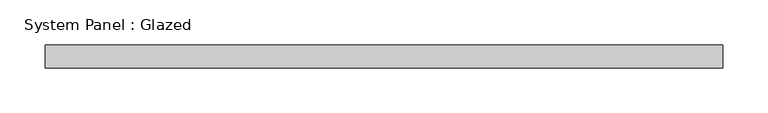
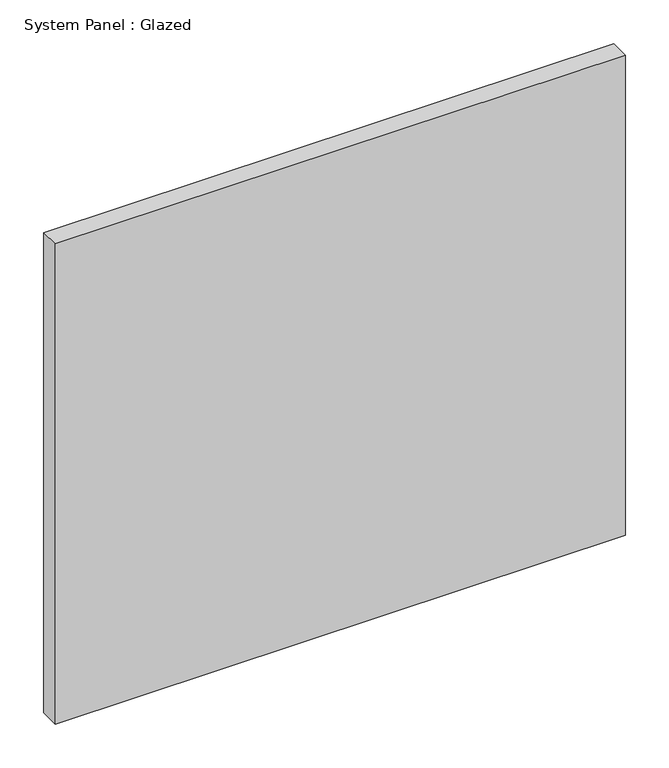
"""IFC4 building model written with IfcOpenShell, lengths in millimetres: plate geometry, System Panel : Glazed."""

from ifc_helpers import new_model, si_unit, origin, origin_with_axes, place, context, project, spatial, polyline, outline, extrude, source, transform, mapped, element, save


def system_panel_glazed_10e47eeb(model_context):
    return source(origin(), model_context, "Body", "SweptSolid", [
        extrude(outline(polyline([(374.658438, 19.05), (-374.658438, 19.05), (-374.658438, 44.45), (374.658438, 44.45), (374.658438, 19.05)])), origin_with_axes(), (0.0, 0.0, 1.0), 666.75),
    ])


if __name__ == "__main__":
    model = new_model("IFC4")
    model_context = context("Model", 3, world=origin())
    ifc_project = project(units=[si_unit("LENGTHUNIT", "METRE", prefix="MILLI")], contexts=[model_context])
    site = spatial("IfcSite", under=ifc_project)
    building = spatial("IfcBuilding", under=site)
    placement = place(None, origin())
    system_panel_glazed_shape = system_panel_glazed_10e47eeb(model_context)
    element("IfcPlate", 1, ObjectType="System Panel : Glazed", at=placement, inside=building, context=model_context, shape_type="MappedRepresentation", body=[
        mapped(system_panel_glazed_shape, transform((0.0, 0.0, 0.0), x_axis=(1.0, 0.0, 0.0), y_axis=(0.0, 1.0, 0.0), z_axis=(0.0, 0.0, 1.0))),
    ])
    save(model, "model.ifc")

# Revit data of these elements
# Type "System Panel : Glazed"
#   Construction Type Id = "GSP4R"
#   Analytic Construction = "1/8 in Pilkington single glazing"
#   Visual Light Transmittance = 0.9
#   Solar Heat Gain Coefficient = 0.86
#   Heat Transfer Coefficient (U) = 1.18115 BTU/(h·ft²·°F)
# Element 1 (IfcPlate, "System Panel : Glazed")
#   Materials on its faces: "Glass"
# Materials
#   "Glass": class "Glass", colour RGB 0 128 192, transparency 0.75, Description = "Soda Lime Glass", Cost = 0
